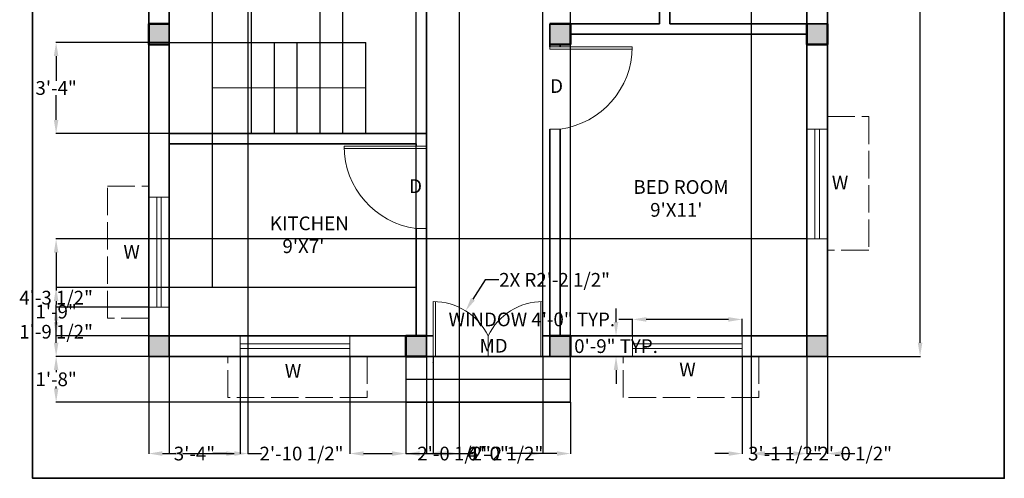
# Model space of a CAD drawing. Units: inches. Extents: x 730 to 1163, y 1530 to 2018.
# Tile 1 of 2: x 732 to 1163, y 1530 to 1731. Entities that reach past the tile are written whole.
import ezdxf

# ---------------------------------------------------------------- set-up
doc = ezdxf.new("R2010")
doc.units = ezdxf.units.IN
doc.header["$MEASUREMENT"] = 0
doc.linetypes.add('ACAD_ISO02W100', pattern=[15, 12, -3])
for name, color, linetype, lineweight in [('A-ANNO-DIMS', 2, 'Continuous', 18), ('A-ANNO-SYMB', 7, 'Continuous', 18), ('A-ANNO-TEXT', 7, 'Continuous', 18), ('A-ANNO-TTLB', 7, 'Continuous', 35), ('A-AREA-IDEN', 7, 'Continuous', 20), ('A-COLS', 7, 'Continuous', 50), ('A-COLS-PATT', 5, 'Continuous', 13), ('A-DOOR', 5, 'Continuous', 18), ('A-FLOR-FIXT', 8, 'Continuous', 18), ('A-FLOR-STRS', 7, 'Continuous', 25), ('A-GLAZ', 5, 'Continuous', 18), ('A-GLAZ-OVHD', 7, 'ACAD_ISO02W100', 13), ('A-WALL', 7, 'Continuous', 35)]:
    doc.layers.add(name, color=color, linetype=linetype, lineweight=lineweight)
doc.styles.get("Standard").update_dxf_attribs({"font": 'arial.ttf'})
doc.dimstyles.get("Standard").update_dxf_attribs({"dimtxt": 6, "dimasz": 6, "dimexe": 0.18, "dimexo": 0.0625, "dimgap": 0.09, "dimtad": 0, "dimtih": 1, "dimtoh": 1, "dimdec": 1, "dimzin": 0, "dimdsep": 46, "dimlunit": 3, "dimtxsty": 'Standard', "dimcen": 0.09, "dimclrt": 1, "dimadec": 0, "dimazin": 0, "dimtfac": 1, "dimtdec": 1, "dimtofl": 0, "dimtmove": 0, "dimatfit": 3, "dimfxl": 1, "dimtolj": 1, "dimtzin": 0, "dimarcsym": 0})

# ---------------------------------------------------------------- blocks, each defined once
blk = doc.blocks.new('*D2')
at = {"layer": 'A-ANNO-DIMS', "color": 0, "lineweight": -2, "transparency": 16777216}
for p, q in [((1085.5, 1964.58), (1126.1, 1964.58)), ((1125.92, 1958.58), (1125.92, 1777.23)), ((1125.92, 1589.58), (1125.92, 1770.92)), ((1085.5, 1583.58), (1126.1, 1583.58))]:
    blk.add_line(p, q, dxfattribs=at)
at = {"layer": 'A-ANNO-DIMS', "color": 0, "transparency": 16777216}
for points in [[(1124.92, 1958.58), (1126.92, 1958.58), (1125.92, 1964.58)], [(1124.92, 1589.58), (1126.92, 1589.58), (1125.92, 1583.58)]]:
    blk.add_solid(points, dxfattribs=at)
at = {"layer": 'Defpoints', "color": 0, "transparency": 16777216}
for p in [(1085.44, 1964.58), (1085.44, 1583.58), (1125.92, 1583.58)]:
    blk.add_point(p, dxfattribs=at)
at = {"layer": 'A-ANNO-DIMS', "color": 0, "transparency": 16777216, "insert": (1125.92, 1774.08), "char_height": 6, "attachment_point": 5}
blk.add_mtext('\\A1;31\'-9.0"', dxfattribs=at)
blk = doc.blocks.new('WINDOW-48IN')
for p, q in [((0, 9), (0, 0)), ((0, 9), (48, 9)), ((48, 0), (48, 9)), ((0, 5.5), (48, 5.5)), ((0, 3.5), (48, 3.5)), ((0, 0), (48, 0))]:
    blk.add_line(p, q)
blk = doc.blocks.new('DOOR-SWING-36IN')
for p, q in [((36, 37), (31.5, 37)), ((0, 2), (36, 2)), ((36, 1), (0, 1)), ((0, 1), (36, 1)), ((36, 0), (36, 2))]:
    blk.add_line(p, q)
blk.add_arc((36.32, 1), 36.32, 97.6281, 180)
blk = doc.blocks.new('*D7')
at = {"layer": 'A-ANNO-DIMS', "color": 0, "lineweight": -2, "transparency": 16777216}
for p, q in [((1000.1, 1599.78), (994.1, 1599.78)), ((1000.1, 1592.64), (1000.1, 1599.96)), ((1042.1, 1599.78), (1006.1, 1599.78)), ((1048.1, 1592.64), (1048.1, 1599.96))]:
    blk.add_line(p, q, dxfattribs=at)
at = {"layer": 'A-ANNO-DIMS', "color": 0, "transparency": 16777216}
for points in [[(1006.1, 1600.78), (1006.1, 1598.78), (1000.1, 1599.78)], [(1042.1, 1600.78), (1042.1, 1598.78), (1048.1, 1599.78)]]:
    blk.add_solid(points, dxfattribs=at)
at = {"layer": 'Defpoints', "color": 0, "transparency": 16777216}
for p in [(1000.1, 1599.78), (1000.1, 1592.58), (1048.1, 1592.58)]:
    blk.add_point(p, dxfattribs=at)
at = {"layer": 'A-ANNO-DIMS', "color": 1, "transparency": 16777216, "insert": (956.05, 1599.78), "char_height": 6, "attachment_point": 5}
blk.add_mtext('\\A1;WINDOW 4\'-0" TYP.', dxfattribs=at)
blk = doc.blocks.new('*D8')
at = {"layer": 'A-ANNO-DIMS', "color": 0, "lineweight": -2, "transparency": 16777216}
for p, q in [((992.9, 1598.58), (992.9, 1604.58)), ((1000.04, 1592.58), (992.72, 1592.58)), ((1000.04, 1583.58), (992.72, 1583.58)), ((992.9, 1577.58), (992.9, 1571.58))]:
    blk.add_line(p, q, dxfattribs=at)
at = {"layer": 'A-ANNO-DIMS', "color": 0, "transparency": 16777216}
for points in [[(991.9, 1598.58), (993.9, 1598.58), (992.9, 1592.58)], [(991.9, 1577.58), (993.9, 1577.58), (992.9, 1583.58)]]:
    blk.add_solid(points, dxfattribs=at)
at = {"layer": 'Defpoints', "color": 0, "transparency": 16777216}
for p in [(1000.1, 1592.58), (992.9, 1583.58), (1000.1, 1583.58)]:
    blk.add_point(p, dxfattribs=at)
at = {"layer": 'A-ANNO-DIMS', "color": 1, "transparency": 16777216, "insert": (992.9, 1588.08), "char_height": 6, "attachment_point": 5}
blk.add_mtext('\\A1;0\'-9" TYP.', dxfattribs=at)
blk = doc.blocks.new('*D15')
at = {"layer": 'A-ANNO-DIMS', "color": 0, "lineweight": -2, "transparency": 16777216}
for p, q in [((797.44, 1964.51), (797.44, 1540.9)), ((831.86, 1955.51), (831.86, 1540.9)), ((803.44, 1541.08), (825.86, 1541.08)), ((831.86, 1541.08), (837.86, 1541.08))]:
    blk.add_line(p, q, dxfattribs=at)
at = {"layer": 'A-ANNO-DIMS', "color": 0, "transparency": 16777216}
for points in [[(803.44, 1542.08), (803.44, 1540.08), (797.44, 1541.08)], [(825.86, 1542.08), (825.86, 1540.08), (831.86, 1541.08)]]:
    blk.add_solid(points, dxfattribs=at)
at = {"layer": 'Defpoints', "color": 0, "transparency": 16777216}
for p in [(797.44, 1964.58), (831.86, 1955.58), (831.86, 1541.08)]:
    blk.add_point(p, dxfattribs=at)
at = {"layer": 'A-ANNO-DIMS', "color": 1, "transparency": 16777216, "insert": (855.3, 1541.08), "char_height": 6, "attachment_point": 5}
blk.add_mtext('\\A1;2\'-10 1/2"', dxfattribs=at)
blk = doc.blocks.new('*D16')
at = {"layer": 'A-ANNO-DIMS', "color": 0, "lineweight": -2, "transparency": 16777216}
for p, q in [((909.94, 1964.51), (909.94, 1540.9)), ((924.22, 1964.51), (924.22, 1540.9)), ((915.94, 1541.08), (918.22, 1541.08)), ((924.22, 1541.08), (930.22, 1541.08))]:
    blk.add_line(p, q, dxfattribs=at)
at = {"layer": 'A-ANNO-DIMS', "color": 0, "transparency": 16777216}
for points in [[(915.94, 1542.08), (915.94, 1540.08), (909.94, 1541.08)], [(918.22, 1542.08), (918.22, 1540.08), (924.22, 1541.08)]]:
    blk.add_solid(points, dxfattribs=at)
at = {"layer": 'Defpoints', "color": 0, "transparency": 16777216}
for p in [(909.94, 1964.58), (924.22, 1964.58), (924.22, 1541.08)]:
    blk.add_point(p, dxfattribs=at)
at = {"layer": 'A-ANNO-DIMS', "color": 1, "transparency": 16777216, "insert": (944.99, 1541.08), "char_height": 6, "attachment_point": 5}
blk.add_mtext('\\A1;1\'-2 1/2"', dxfattribs=at)
blk = doc.blocks.new('*D17')
at = {"layer": 'A-ANNO-DIMS', "color": 0, "lineweight": -2, "transparency": 16777216}
for p, q in [((1076.44, 1964.51), (1076.44, 1540.9)), ((1052.04, 1955.51), (1052.04, 1540.9)), ((1058.04, 1541.08), (1070.44, 1541.08)), ((1076.44, 1541.08), (1082.44, 1541.08))]:
    blk.add_line(p, q, dxfattribs=at)
at = {"layer": 'A-ANNO-DIMS', "color": 0, "transparency": 16777216}
for points in [[(1058.04, 1542.08), (1058.04, 1540.08), (1052.04, 1541.08)], [(1070.44, 1542.08), (1070.44, 1540.08), (1076.44, 1541.08)]]:
    blk.add_solid(points, dxfattribs=at)
at = {"layer": 'Defpoints', "color": 0, "transparency": 16777216}
for p in [(1076.44, 1964.58), (1052.04, 1955.58), (1076.44, 1541.08)]:
    blk.add_point(p, dxfattribs=at)
at = {"layer": 'A-ANNO-DIMS', "color": 1, "transparency": 16777216, "insert": (1097.55, 1541.08), "char_height": 6, "attachment_point": 5}
blk.add_mtext('\\A1;2\'-0 1/2"', dxfattribs=at)
blk = doc.blocks.new('*D20')
at = {"layer": 'A-ANNO-DIMS', "color": 0, "lineweight": -2, "transparency": 16777216}
for p, q in [((788.38, 1605.2), (747.76, 1605.2)), ((747.94, 1599.2), (747.94, 1597.58)), ((747.94, 1589.58), (747.94, 1591.2)), ((788.38, 1583.58), (747.76, 1583.58))]:
    blk.add_line(p, q, dxfattribs=at)
at = {"layer": 'A-ANNO-DIMS', "color": 0, "transparency": 16777216}
for points in [[(746.94, 1599.2), (748.94, 1599.2), (747.94, 1605.2)], [(746.94, 1589.58), (748.94, 1589.58), (747.94, 1583.58)]]:
    blk.add_solid(points, dxfattribs=at)
at = {"layer": 'Defpoints', "color": 0, "transparency": 16777216}
for p in [(788.44, 1605.2), (747.94, 1583.58), (788.44, 1583.58)]:
    blk.add_point(p, dxfattribs=at)
at = {"layer": 'A-ANNO-DIMS', "color": 1, "transparency": 16777216, "insert": (747.94, 1594.39), "char_height": 6, "attachment_point": 5}
blk.add_mtext('\\A1;1\'-9 1/2"', dxfattribs=at)
blk = doc.blocks.new('*D23')
at = {"layer": 'A-ANNO-DIMS', "color": 0, "lineweight": -2, "transparency": 16777216}
for p, q in [((1076.38, 1635), (747.76, 1635)), ((747.94, 1629), (747.94, 1612.48)), ((747.94, 1589.58), (747.94, 1606.09)), ((1085.38, 1583.58), (747.76, 1583.58))]:
    blk.add_line(p, q, dxfattribs=at)
at = {"layer": 'A-ANNO-DIMS', "color": 0, "transparency": 16777216}
for points in [[(746.94, 1629), (748.94, 1629), (747.94, 1635)], [(746.94, 1589.58), (748.94, 1589.58), (747.94, 1583.58)]]:
    blk.add_solid(points, dxfattribs=at)
at = {"layer": 'Defpoints', "color": 0, "transparency": 16777216}
for p in [(1076.44, 1635), (747.94, 1583.58), (1085.44, 1583.58)]:
    blk.add_point(p, dxfattribs=at)
at = {"layer": 'A-ANNO-DIMS', "color": 1, "transparency": 16777216, "insert": (747.94, 1609.29), "char_height": 6, "attachment_point": 5}
blk.add_mtext('\\A1;4\'-3 1/2"', dxfattribs=at)
blk = doc.blocks.new('*D24')
at = {"layer": 'A-ANNO-DIMS', "color": 0, "lineweight": -2, "transparency": 16777216}
for p, q in [((788.44, 1583.51), (788.44, 1540.9)), ((828.47, 1583.51), (828.47, 1540.9)), ((794.44, 1541.08), (800.39, 1541.08)), ((822.47, 1541.08), (816.52, 1541.08))]:
    blk.add_line(p, q, dxfattribs=at)
at = {"layer": 'A-ANNO-DIMS', "color": 0, "transparency": 16777216}
for points in [[(794.44, 1542.08), (794.44, 1540.08), (788.44, 1541.08)], [(822.47, 1542.08), (822.47, 1540.08), (828.47, 1541.08)]]:
    blk.add_solid(points, dxfattribs=at)
at = {"layer": 'Defpoints', "color": 0, "transparency": 16777216}
for p in [(788.44, 1583.58), (828.47, 1583.58), (828.47, 1541.08)]:
    blk.add_point(p, dxfattribs=at)
at = {"layer": 'A-ANNO-DIMS', "color": 1, "transparency": 16777216, "insert": (808.45, 1541.08), "char_height": 6, "attachment_point": 5}
blk.add_mtext('\\A1;3\'-4"', dxfattribs=at)
blk = doc.blocks.new('*D25')
at = {"layer": 'A-ANNO-DIMS', "color": 0, "lineweight": -2, "transparency": 16777216}
for p, q in [((1048.102774, 1583.514415), (1048.102774, 1540.896915)), ((1085.442098, 1583.514415), (1085.442098, 1540.896915)), ((1042.102774, 1541.076915), (1036.102774, 1541.076915)), ((1091.442098, 1541.076915), (1097.442098, 1541.076915))]:
    blk.add_line(p, q, dxfattribs=at)
at = {"layer": 'A-ANNO-DIMS', "color": 0, "transparency": 16777216}
for points in [[(1042.102774, 1542.076915), (1042.102774, 1540.076915), (1048.102774, 1541.076915)], [(1091.442098, 1542.076915), (1091.442098, 1540.076915), (1085.442098, 1541.076915)]]:
    blk.add_solid(points, dxfattribs=at)
at = {"layer": 'Defpoints', "color": 0, "transparency": 16777216}
for p in [(1048.102774, 1583.576915), (1085.442098, 1583.576915), (1085.442098, 1541.076915)]:
    blk.add_point(p, dxfattribs=at)
at = {"layer": 'A-ANNO-DIMS', "color": 1, "transparency": 16777216, "insert": (1066.772436, 1541.076915), "char_height": 6, "attachment_point": 5}
blk.add_mtext('\\A1;3\'-1 1/2"', dxfattribs=at)
blk = doc.blocks.new('*D26')
at = {"layer": 'A-ANNO-DIMS', "color": 0, "lineweight": -2, "transparency": 16777216}
for p, q in [((912.94, 1583.51), (912.94, 1540.9)), ((960.94, 1583.51), (960.94, 1540.9)), ((918.94, 1541.08), (928.76, 1541.08)), ((954.94, 1541.08), (945.13, 1541.08))]:
    blk.add_line(p, q, dxfattribs=at)
at = {"layer": 'A-ANNO-DIMS', "color": 0, "transparency": 16777216}
for points in [[(918.94, 1542.08), (918.94, 1540.08), (912.94, 1541.08)], [(954.94, 1542.08), (954.94, 1540.08), (960.94, 1541.08)]]:
    blk.add_solid(points, dxfattribs=at)
at = {"layer": 'Defpoints', "color": 0, "transparency": 16777216}
for p in [(912.94, 1583.58), (960.94, 1583.58), (960.94, 1541.08)]:
    blk.add_point(p, dxfattribs=at)
at = {"layer": 'A-ANNO-DIMS', "color": 1, "transparency": 16777216, "insert": (936.94, 1541.08), "char_height": 6, "attachment_point": 5}
blk.add_mtext('\\A1;4\'-0"', dxfattribs=at)
blk = doc.blocks.new('*D28')
at = {"layer": 'A-ANNO-DIMS', "color": 0, "lineweight": -2, "transparency": 16777216}
for p, q in [((857.44, 2005.08), (851.44, 2005.08)), ((863.44, 1721.06), (863.44, 2005.26)), ((873.44, 1721.06), (873.44, 2005.26)), ((879.44, 2005.08), (885.44, 2005.08))]:
    blk.add_line(p, q, dxfattribs=at)
at = {"layer": 'A-ANNO-DIMS', "color": 0, "transparency": 16777216}
for points in [[(857.44, 2006.08), (857.44, 2004.08), (863.44, 2005.08)], [(879.44, 2006.08), (879.44, 2004.08), (873.44, 2005.08)]]:
    blk.add_solid(points, dxfattribs=at)
at = {"layer": 'Defpoints', "color": 0, "transparency": 16777216}
for p in [(873.44, 2005.08), (863.44, 1721), (873.44, 1721)]:
    blk.add_point(p, dxfattribs=at)
at = {"layer": 'A-ANNO-DIMS', "color": 1, "transparency": 16777216, "insert": (895.84, 2005.08), "char_height": 6, "attachment_point": 5}
blk.add_mtext('\\A1;0\'-10"', dxfattribs=at)
blk = doc.blocks.new('*D29')
at = {"layer": 'A-ANNO-DIMS', "color": 0, "lineweight": -2, "transparency": 16777216}
for p, q in [((797.38, 1721), (747.76, 1721)), ((747.94, 1715), (747.94, 1704.19)), ((747.94, 1687.08), (747.94, 1697.88)), ((797.38, 1681.08), (747.76, 1681.08))]:
    blk.add_line(p, q, dxfattribs=at)
at = {"layer": 'A-ANNO-DIMS', "color": 0, "transparency": 16777216}
for points in [[(746.94, 1715), (748.94, 1715), (747.94, 1721)], [(746.94, 1687.08), (748.94, 1687.08), (747.94, 1681.08)]]:
    blk.add_solid(points, dxfattribs=at)
at = {"layer": 'Defpoints', "color": 0, "transparency": 16777216}
for p in [(747.94, 1721), (797.44, 1721), (797.44, 1681.08)]:
    blk.add_point(p, dxfattribs=at)
at = {"layer": 'A-ANNO-DIMS', "color": 1, "transparency": 16777216, "insert": (747.94, 1701.04), "char_height": 6, "attachment_point": 5}
blk.add_mtext('\\A1;3\'-4"', dxfattribs=at)
blk = doc.blocks.new('*D30')
at = {"layer": 'A-ANNO-DIMS', "color": 0, "lineweight": -2, "transparency": 16777216}
for p, q in [((900.94, 1563.51), (900.94, 1540.9)), ((973.01, 1563.51), (973.01, 1540.9)), ((906.94, 1541.08), (928.89, 1541.08)), ((967.01, 1541.08), (945.06, 1541.08))]:
    blk.add_line(p, q, dxfattribs=at)
at = {"layer": 'A-ANNO-DIMS', "color": 0, "transparency": 16777216}
for points in [[(906.94, 1542.08), (906.94, 1540.08), (900.94, 1541.08)], [(967.01, 1542.08), (967.01, 1540.08), (973.01, 1541.08)]]:
    blk.add_solid(points, dxfattribs=at)
at = {"layer": 'Defpoints', "color": 0, "transparency": 16777216}
for p in [(900.94, 1563.58), (973.01, 1563.58), (973.01, 1541.08)]:
    blk.add_point(p, dxfattribs=at)
at = {"layer": 'A-ANNO-DIMS', "color": 1, "transparency": 16777216, "insert": (936.98, 1541.08), "char_height": 6, "attachment_point": 5}
blk.add_mtext('\\A1;6\'-0"', dxfattribs=at)
blk = doc.blocks.new('*D31')
at = {"layer": 'A-ANNO-DIMS', "color": 0, "lineweight": -2, "transparency": 16777216}
for p, q in [((972.88, 1583.58), (747.76, 1583.58)), ((747.94, 1577.58), (747.94, 1576.73)), ((747.94, 1569.58), (747.94, 1570.42)), ((972.95, 1563.58), (747.76, 1563.58))]:
    blk.add_line(p, q, dxfattribs=at)
at = {"layer": 'A-ANNO-DIMS', "color": 0, "transparency": 16777216}
for points in [[(746.94, 1577.58), (748.94, 1577.58), (747.94, 1583.58)], [(746.94, 1569.58), (748.94, 1569.58), (747.94, 1563.58)]]:
    blk.add_solid(points, dxfattribs=at)
at = {"layer": 'Defpoints', "color": 0, "transparency": 16777216}
for p in [(747.94, 1583.58), (972.94, 1583.58), (973.01, 1563.58)]:
    blk.add_point(p, dxfattribs=at)
at = {"layer": 'A-ANNO-DIMS', "color": 1, "transparency": 16777216, "insert": (747.94, 1573.58), "char_height": 6, "attachment_point": 5}
blk.add_mtext('\\A1;1\'-8"', dxfattribs=at)
blk = doc.blocks.new('*D32')
at = {"layer": 'A-ANNO-DIMS', "color": 0, "lineweight": -2, "transparency": 16777216}
for p, q in [((791.44, 2005.08), (785.44, 2005.08)), ((797.44, 1605.26), (797.44, 2005.26)), ((816.4, 1613.85), (816.4, 2005.26)), ((822.4, 2005.08), (828.4, 2005.08))]:
    blk.add_line(p, q, dxfattribs=at)
at = {"layer": 'A-ANNO-DIMS', "color": 0, "transparency": 16777216}
for points in [[(791.44, 2006.08), (791.44, 2004.08), (797.44, 2005.08)], [(822.4, 2006.08), (822.4, 2004.08), (816.4, 2005.08)]]:
    blk.add_solid(points, dxfattribs=at)
at = {"layer": 'Defpoints', "color": 0, "transparency": 16777216}
for p in [(816.4, 2005.08), (816.4, 1613.79), (797.44, 1605.2)]:
    blk.add_point(p, dxfattribs=at)
at = {"layer": 'A-ANNO-DIMS', "color": 1, "transparency": 16777216, "insert": (806.92, 2005.08), "char_height": 6, "attachment_point": 5}
blk.add_mtext('\\A1;1\'-7"', dxfattribs=at)
blk = doc.blocks.new('*D33')
at = {"layer": 'A-ANNO-DIMS', "color": 0, "lineweight": -2, "transparency": 16777216}
for p, q in [((905.38, 1613.79), (747.76, 1613.79)), ((747.94, 1607.79), (747.94, 1606.34)), ((747.94, 1598.58), (747.94, 1600.03)), ((905.38, 1592.58), (747.76, 1592.58))]:
    blk.add_line(p, q, dxfattribs=at)
at = {"layer": 'A-ANNO-DIMS', "color": 0, "transparency": 16777216}
for points in [[(746.94, 1607.79), (748.94, 1607.79), (747.94, 1613.79)], [(746.94, 1598.58), (748.94, 1598.58), (747.94, 1592.58)]]:
    blk.add_solid(points, dxfattribs=at)
at = {"layer": 'Defpoints', "color": 0, "transparency": 16777216}
for p in [(747.94, 1613.79), (905.44, 1613.79), (905.44, 1592.58)]:
    blk.add_point(p, dxfattribs=at)
at = {"layer": 'A-ANNO-DIMS', "color": 1, "transparency": 16777216, "insert": (747.94, 1603.18), "char_height": 6, "attachment_point": 5}
blk.add_mtext('\\A1;1\'-9"', dxfattribs=at)
blk = doc.blocks.new('*D34')
at = {"layer": 'A-ANNO-DIMS', "color": 0, "lineweight": -2, "transparency": 16777216}
for p, q in [((899.44, 2005.08), (893.44, 2005.08)), ((905.44, 1592.64), (905.44, 2005.26)), ((909.94, 1592.64), (909.94, 2005.26)), ((915.94, 2005.08), (921.94, 2005.08))]:
    blk.add_line(p, q, dxfattribs=at)
at = {"layer": 'A-ANNO-DIMS', "color": 0, "transparency": 16777216}
for points in [[(899.44, 2006.08), (899.44, 2004.08), (905.44, 2005.08)], [(915.94, 2006.08), (915.94, 2004.08), (909.94, 2005.08)]]:
    blk.add_solid(points, dxfattribs=at)
at = {"layer": 'Defpoints', "color": 0, "transparency": 16777216}
for p in [(909.94, 2005.08), (905.44, 1592.58), (909.94, 1592.58)]:
    blk.add_point(p, dxfattribs=at)
at = {"layer": 'A-ANNO-DIMS', "color": 1, "transparency": 16777216, "insert": (937, 2005.08), "char_height": 6, "attachment_point": 5}
blk.add_mtext('\\A1;0\'-4 1/2"', dxfattribs=at)
blk = doc.blocks.new('*D35')
at = {"layer": 'A-ANNO-DIMS', "color": 0, "lineweight": -2, "transparency": 16777216}
for p, q in [((876.47, 1583.51), (876.47, 1540.9)), ((900.94, 1563.51), (900.94, 1540.9)), ((882.47, 1541.08), (894.94, 1541.08)), ((900.94, 1541.08), (906.94, 1541.08))]:
    blk.add_line(p, q, dxfattribs=at)
at = {"layer": 'A-ANNO-DIMS', "color": 0, "transparency": 16777216}
for points in [[(882.47, 1542.08), (882.47, 1540.08), (876.47, 1541.08)], [(894.94, 1542.08), (894.94, 1540.08), (900.94, 1541.08)]]:
    blk.add_solid(points, dxfattribs=at)
at = {"layer": 'Defpoints', "color": 0, "transparency": 16777216}
for p in [(876.47, 1583.58), (900.94, 1563.58), (900.94, 1541.08)]:
    blk.add_point(p, dxfattribs=at)
at = {"layer": 'A-ANNO-DIMS', "color": 1, "transparency": 16777216, "insert": (922.05, 1541.08), "char_height": 6, "attachment_point": 5}
blk.add_mtext('\\A1;2\'-0 1/2"', dxfattribs=at)
blk = doc.blocks.new('*D36')
at = {"layer": 'A-ANNO-DIMS', "color": 0, "lineweight": -2, "transparency": 16777216}
for p, q in [((954.94, 2005.08), (948.94, 2005.08)), ((960.94, 1583.64), (960.94, 2005.26)), ((972.94, 1583.64), (972.94, 2005.26)), ((978.94, 2005.08), (984.94, 2005.08))]:
    blk.add_line(p, q, dxfattribs=at)
at = {"layer": 'A-ANNO-DIMS', "color": 0, "transparency": 16777216}
for points in [[(954.94, 2006.08), (954.94, 2004.08), (960.94, 2005.08)], [(978.94, 2006.08), (978.94, 2004.08), (972.94, 2005.08)]]:
    blk.add_solid(points, dxfattribs=at)
at = {"layer": 'Defpoints', "color": 0, "transparency": 16777216}
for p in [(972.94, 2005.08), (960.94, 1583.58), (972.94, 1583.58)]:
    blk.add_point(p, dxfattribs=at)
at = {"layer": 'A-ANNO-DIMS', "color": 1, "transparency": 16777216, "insert": (992.72, 2005.08), "char_height": 6, "attachment_point": 5}
blk.add_mtext('\\A1;1\'-0"', dxfattribs=at)
blk = doc.blocks.new('*D39')
at = {"layer": 'A-ANNO-DIMS', "color": 0, "lineweight": -2, "transparency": 16777216}
for p, q in [((935.58, 1617.1), (930.27, 1608.61)), ((941.58, 1617.1), (935.58, 1617.1)), ((912.94, 1580.79), (912.94, 1580.97)), ((912.85, 1580.88), (913.03, 1580.88))]:
    blk.add_line(p, q, dxfattribs=at)
at = {"layer": 'A-ANNO-DIMS', "color": 0, "transparency": 16777216}
blk.add_solid([(929.43, 1609.14), (931.12, 1608.08), (927.09, 1603.52)], dxfattribs=at)
at = {"layer": 'Defpoints', "color": 0, "transparency": 16777216}
for p in [(927.09, 1603.52), (912.94, 1580.88)]:
    blk.add_point(p, dxfattribs=at)
at = {"layer": 'A-ANNO-DIMS', "color": 1, "transparency": 16777216, "insert": (966.01, 1617.1), "char_height": 6, "attachment_point": 5}
blk.add_mtext('\\A1;2X R2\'-2 1/2"', dxfattribs=at)

msp = doc.modelspace()

# ---------------------------------------------------------------- hatches: boundary and pattern name
at = {"layer": 'A-COLS-PATT'}
h = msp.add_hatch(color=256, dxfattribs=at)
h.dxf.hatch_style = 1
h.paths.add_polyline_path([(797.44, 1964.58), (788.44, 1964.58), (788.44, 1955.58), (797.44, 1955.58)])
h.paths.add_polyline_path([(909.94, 1964.58), (900.94, 1964.58), (900.94, 1955.58), (909.94, 1955.58)])
h.paths.add_polyline_path([(972.94, 1964.58), (963.94, 1964.58), (963.94, 1955.58), (972.94, 1955.58)])
h.paths.add_polyline_path([(1085.44, 1964.58), (1076.44, 1964.58), (1076.44, 1955.58), (1085.44, 1955.58)])
h.paths.add_polyline_path([(797.44, 1828.08), (788.44, 1828.08), (788.44, 1819.08), (797.44, 1819.08)])
h.paths.add_polyline_path([(909.94, 1828.08), (900.94, 1828.08), (900.94, 1819.08), (909.94, 1819.08)])
h.paths.add_polyline_path([(972.94, 1828.08), (963.94, 1828.08), (963.94, 1819.08), (972.94, 1819.08)])
h.paths.add_polyline_path([(1085.44, 1828.08), (1076.44, 1828.08), (1076.44, 1819.08), (1085.44, 1819.08)])
h.paths.add_polyline_path([(797.44, 1729.08), (788.44, 1729.08), (788.44, 1720.08), (797.44, 1720.08)])
h.paths.add_polyline_path([(972.96, 1729.08), (963.94, 1729.08), (963.94, 1720.07), (972.96, 1720.07)])
h.paths.add_polyline_path([(1085.44, 1729.08), (1076.44, 1729.08), (1076.44, 1720.08), (1085.44, 1720.08)])
h.paths.add_polyline_path([(1085.44, 1592.58), (1076.44, 1592.58), (1076.44, 1583.58), (1085.44, 1583.58)])
h.paths.add_polyline_path([(972.94, 1592.58), (963.94, 1592.58), (963.94, 1583.58), (972.94, 1583.58)])
h.paths.add_polyline_path([(909.94, 1592.58), (900.94, 1592.58), (900.94, 1583.58), (909.94, 1583.58)])
h.paths.add_polyline_path([(797.44, 1592.58), (788.44, 1592.58), (788.44, 1583.58), (797.44, 1583.58)])

# ---------------------------------------------------------------- linework, layer by layer
at = {"layer": 'A-ANNO-SYMB'}
for p, q in [((816.36, 1701.04), (816.36, 1745.67)), ((883.44, 1701.04), (816.36, 1701.04))]:
    msp.add_line(p, q, dxfattribs=at)
at = {"layer": 'A-ANNO-TTLB'}
msp.add_lwpolyline([(737.62, 2017.92), (1162.77, 2017.92), (1162.77, 1530.25), (737.62, 1530.25)], close=True, dxfattribs=at)
at = {"layer": 'A-COLS'}
for p, q in [((788.44, 1729.08), (797.44, 1729.08)), ((788.44, 1729.08), (788.44, 1720.08)), ((963.94, 1729.08), (972.96, 1729.08)), ((972.96, 1729.08), (972.96, 1720.07)), ((1076.44, 1729.08), (1076.44, 1720.08)), ((1085.44, 1720.08), (1085.44, 1729.08)), ((788.44, 1720.08), (797.44, 1720.08)), ((972.96, 1720.07), (963.94, 1720.07)), ((1076.44, 1720.08), (1085.44, 1720.08)), ((909.94, 1592.58), (900.94, 1592.58)), ((900.94, 1592.58), (900.94, 1583.58)), ((963.94, 1592.58), (972.94, 1592.58)), ((972.94, 1592.58), (972.94, 1583.58)), ((900.94, 1583.58), (909.94, 1583.58))]:
    msp.add_line(p, q, dxfattribs=at)
at = {"layer": 'A-DOOR'}
for p, q in [((912.94, 1583.58), (912.94, 1607.58)), ((912.94, 1607.58), (912.94, 1583.58)), ((913.94, 1607.58), (913.94, 1583.58)), ((959.94, 1607.58), (959.94, 1583.58)), ((960.94, 1583.58), (960.94, 1607.58)), ((960.94, 1607.58), (960.94, 1583.58)), ((936.94, 1583.58), (936.94, 1592.58)), ((909.94, 1583.58), (912.94, 1583.58)), ((912.94, 1583.58), (960.94, 1583.58)), ((960.94, 1583.58), (936.94, 1583.58))]:
    msp.add_line(p, q, dxfattribs=at)
for centre, start, end in [((912.94, 1580.88), 25.9892, 90), ((960.94, 1580.88), 90, 154.0108)]:
    msp.add_arc(centre, 26.7, start, end, dxfattribs=at)
at = {"layer": 'A-FLOR-FIXT'}
for p, q in [((816.4, 1676.58), (816.4, 1613.79)), ((816.4, 1613.79), (905.44, 1613.79))]:
    msp.add_line(p, q, dxfattribs=at)
at = {"layer": 'A-FLOR-STRS'}
for p, q in [((833.44, 1681.08), (833.44, 1783.08)), ((797.44, 1685), (797.44, 1721)), ((797.44, 1721), (883.44, 1721)), ((843.44, 1681.08), (843.44, 1721)), ((853.44, 1681.08), (853.44, 1721)), ((863.44, 1681.08), (863.44, 1721)), ((873.44, 1681.08), (873.44, 1721)), ((883.44, 1681.08), (883.44, 1721)), ((797.44, 1681.08), (833.44, 1681.08)), ((900.94, 1583.58), (900.94, 1563.58)), ((973.01, 1563.58), (973.01, 1583.58)), ((900.94, 1573.58), (973.01, 1573.58)), ((900.94, 1563.58), (973.01, 1563.58))]:
    msp.add_line(p, q, dxfattribs=at)
at = {"layer": 'A-GLAZ-OVHD'}
for p, q in [((1085.44, 1688.5), (1103.44, 1688.5)), ((1103.44, 1688.5), (1103.44, 1630.14)), ((770.44, 1600.35), (770.44, 1658.07)), ((770.44, 1658.07), (788.44, 1658.07)), ((1103.44, 1630.14), (1085.44, 1630.14)), ((788.44, 1600.35), (770.44, 1600.35)), ((823.03, 1565.58), (823.03, 1583.58)), ((884.03, 1583.58), (884.03, 1565.58)), ((996.05, 1565.58), (996.05, 1583.58)), ((1055.4, 1583.58), (1055.4, 1565.58)), ((884.03, 1565.58), (823.03, 1565.58)), ((1055.4, 1565.58), (996.05, 1565.58))]:
    msp.add_line(p, q, dxfattribs=at)
at = {"layer": 'A-WALL'}
for p, q in [((788.44, 1964.58), (788.44, 1583.58)), ((797.44, 1964.58), (797.44, 1681.08)), ((1076.44, 1964.58), (1076.44, 1583.58)), ((1085.44, 1964.58), (1085.44, 1583.58)), ((1011.94, 1794.08), (1011.94, 1729.08)), ((1016.44, 1794.08), (1016.44, 1729.08)), ((963.94, 1729.08), (963.94, 1719.07)), ((963.94, 1729.08), (1011.94, 1729.08)), ((1016.44, 1729.08), (1085.44, 1729.08)), ((972.96, 1724.58), (1076.44, 1724.58)), ((968.44, 1720.07), (968.44, 1719.07)), ((797.44, 1681.08), (909.94, 1681.08)), ((909.94, 1681.08), (909.94, 1675.58)), ((963.94, 1683.07), (963.94, 1583.58)), ((968.44, 1683.07), (968.44, 1592.58)), ((797.44, 1676.58), (905.44, 1676.58)), ((797.44, 1676.58), (797.44, 1583.58)), ((905.44, 1676.58), (905.44, 1675.58)), ((905.44, 1639.58), (905.44, 1592.58)), ((909.94, 1639.58), (909.94, 1583.58)), ((788.44, 1592.58), (912.94, 1592.58)), ((960.94, 1592.58), (1085.44, 1592.58)), ((788.44, 1583.58), (1085.44, 1583.58))]:
    msp.add_line(p, q, dxfattribs=at)

# ---------------------------------------------------------------- block references
at = {"layer": 'A-DOOR', "rotation": 180}
msp.add_blockref('DOOR-SWING-36IN', (999.94, 1720.07), dxfattribs=at)
at = {"layer": 'A-DOOR', "extrusion": (0, 0, -1), "zscale": -1, "rotation": 180}
msp.add_blockref('DOOR-SWING-36IN', (-873.94, 1676.58), dxfattribs=at)
at = {"layer": 'A-GLAZ'}
for p, rotation in [((1085.44, 1635), 89.999999999999), ((797.44, 1605.2), 89.999999999999), ((876.47, 1592.58), 180), ((1048.1, 1592.58), 180)]:
    msp.add_blockref('WINDOW-48IN', p, dxfattribs=dict(at, rotation=rotation))

# ---------------------------------------------------------------- texts
at = {"layer": 'A-ANNO-TEXT', "char_height": 6, "attachment_point": 1}
for s, width, insert in [('D', 6.6774, (964.07, 1704.89)), ('D', 6.6774, (902.39, 1661.08)), ('W', 10.9415, (1087.31, 1662.65)), ('W', 10.9415, (777.38, 1632.35)), ('MD', 9.1896, (933.19, 1591.26)), ('W', 10.9415, (847.99, 1580.23)), ('W', 10.9415, (1020.57, 1580.86))]:
    msp.add_mtext_dynamic_manual_height_columns(s, width=width, gutter_width=30, heights=[0], dxfattribs=dict(at, insert=insert))
at = {"layer": 'A-AREA-IDEN', "char_height": 6, "attachment_point": 1}
for s, width, insert in [("BED ROOM\\P    9'X11'", 51.376, (1000.5, 1660.72)), ("KITCHEN\\P   9'X7'", 43.6922, (841.46, 1644.81))]:
    msp.add_mtext_dynamic_manual_height_columns(s, width=width, gutter_width=30, heights=[0], dxfattribs=dict(at, insert=insert))

# ---------------------------------------------------------------- dimensions: what is measured, and where the dimension line sits
at = {"layer": 'A-ANNO-DIMS'}
for base, p1, p2, picture, middle in [((909.94, 2005.08), (905.44, 1592.58), (909.94, 1592.58), '*D34', (937, 2005.08)), ((816.4, 2005.08), (797.44, 1605.2), (816.4, 1613.79), '*D32', (806.92, 2005.08)), ((873.44, 2005.08), (863.44, 1721), (873.44, 1721), '*D28', (895.84, 2005.08)), ((972.94, 2005.08), (960.94, 1583.58), (972.94, 1583.58), '*D36', (992.72, 2005.08)), ((831.86, 1541.08), (797.44, 1964.58), (831.86, 1955.58), '*D15', (855.3, 1541.08)), ((924.22, 1541.08), (909.94, 1964.58), (924.22, 1964.58), '*D16', (944.99, 1541.08)), ((1076.44, 1541.08), (1052.04, 1955.58), (1076.44, 1964.58), '*D17', (1097.55, 1541.08)), ((828.47, 1541.08), (788.44, 1583.58), (828.47, 1583.58), '*D24', (808.45, 1541.08)), ((900.94, 1541.08), (876.47, 1583.58), (900.94, 1563.58), '*D35', (922.05, 1541.08)), ((960.94, 1541.08), (912.94, 1583.58), (960.94, 1583.58), '*D26', (936.94, 1541.08)), ((1085.44, 1541.08), (1048.1, 1583.58), (1085.44, 1583.58), '*D25', (1066.77, 1541.08)), ((973.01, 1541.08), (900.94, 1563.58), (973.01, 1563.58), '*D30', (936.98, 1541.08))]:
    dim = msp.add_linear_dim(base=base, p1=p1, p2=p2, dimstyle='Standard', override={"dimdec": 1, "dimlfac": 1, "dimrnd": 0, "dimzin": 1, "dimdsep": 46, "dimlunit": 4, "dimfrac": 2}, dxfattribs=at)
    dim.commit()
    dim.dimension.update_dxf_attribs({"geometry": picture, "text_midpoint": middle})
dim = msp.add_linear_dim(base=(1125.92, 1583.58), p1=(1085.44, 1964.58), p2=(1085.44, 1583.58), angle=90, dimstyle='Standard', override={"dimclrd": 0, "dimclre": 0, "dimclrt": 0}, dxfattribs=at)
dim.commit()
dim.dimension.update_dxf_attribs({"geometry": '*D2', "text_midpoint": (1125.92, 1774.08), "dimtype": 160})
for base, p1, p2, picture, middle in [((747.94, 1721), (797.44, 1681.08), (797.44, 1721), '*D29', (747.94, 1701.04)), ((747.94, 1583.58), (1076.44, 1635), (1085.44, 1583.58), '*D23', (747.94, 1609.29)), ((747.94, 1613.79), (905.44, 1592.58), (905.44, 1613.79), '*D33', (747.94, 1603.18)), ((747.94, 1583.58), (788.44, 1605.2), (788.44, 1583.58), '*D20', (747.94, 1594.39)), ((747.94, 1583.58), (973.01, 1563.58), (972.94, 1583.58), '*D31', (747.94, 1573.58))]:
    dim = msp.add_linear_dim(base=base, p1=p1, p2=p2, angle=90, dimstyle='Standard', override={"dimdec": 1, "dimlfac": 1, "dimrnd": 0, "dimzin": 1, "dimdsep": 46, "dimlunit": 4, "dimfrac": 2}, dxfattribs=at)
    dim.commit()
    dim.dimension.update_dxf_attribs({"geometry": picture, "text_midpoint": middle})
dim = msp.add_radius_dim(center=(912.94, 1580.88), mpoint=(927.09, 1603.52), text='2X <>', dimstyle='Standard', override={"dimdec": 1, "dimlfac": 1, "dimrnd": 0, "dimzin": 1, "dimdsep": 46, "dimlunit": 4, "dimfrac": 2}, dxfattribs=at)
dim.commit()
dim.dimension.update_dxf_attribs({"geometry": '*D39', "text_midpoint": (966.01, 1617.1), "dimtype": 164})
for base, p1, p2, angle, text, picture, middle in [((1000.1, 1599.78), (1048.1, 1592.58), (1000.1, 1592.58), 180, 'WINDOW <> TYP.', '*D7', (956.05, 1599.78)), ((992.9, 1583.58), (1000.1, 1592.58), (1000.1, 1583.58), 270, '<> TYP.', '*D8', (992.9, 1588.08))]:
    dim = msp.add_linear_dim(base=base, p1=p1, p2=p2, angle=angle, text=text, dimstyle='Standard', override={"dimdec": 1, "dimlfac": 1, "dimrnd": 0, "dimzin": 1, "dimdsep": 46, "dimlunit": 4, "dimfrac": 2}, dxfattribs=at)
    dim.commit()
    dim.dimension.update_dxf_attribs({"geometry": picture, "text_midpoint": middle})

doc.saveas('drawing.dxf')
